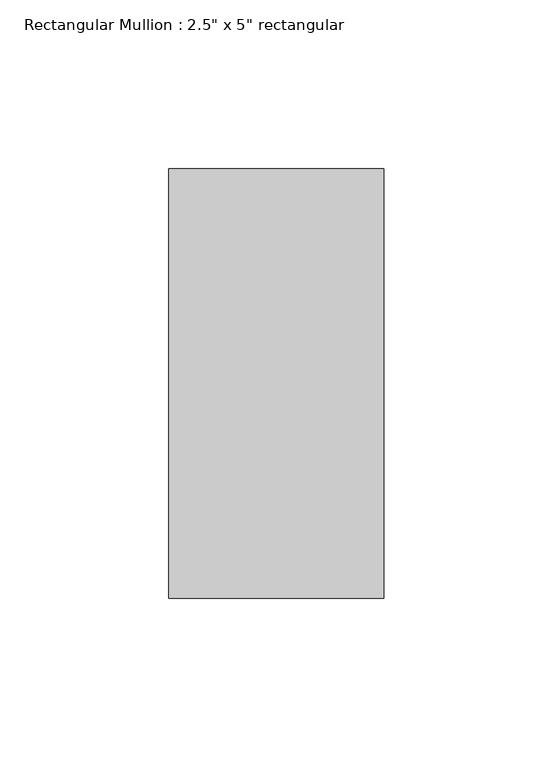
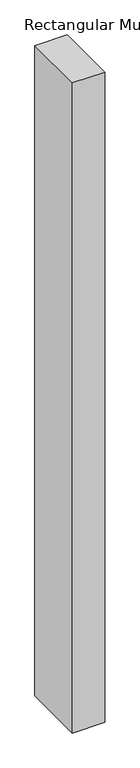
"""IFC4 building model written with IfcOpenShell, lengths in millimetres: member geometry."""

from ifc_helpers import new_model, si_unit, frame, origin, place, context, project, spatial, polyline, outline, extrude, source, transform, mapped, element, save


def member_488afbc6(model_context):
    return source(origin(), model_context, "Body", "SweptSolid", [
        extrude(outline(polyline([(31.75, 63.5), (31.75, -63.5), (-31.75, -63.5), (-31.75, 63.5), (31.75, 63.5)])), frame((0.0, 0.0, -1343.8279521), z_axis=(0.0, 0.0, 1.0), x_axis=(1.0, 0.0, 0.0)), (0.0, 0.0, 1.0), 1343.8279521),
    ])


if __name__ == "__main__":
    model = new_model("IFC4")
    model_context = context("Model", 3, world=origin())
    ifc_project = project(units=[si_unit("LENGTHUNIT", "METRE", prefix="MILLI")], contexts=[model_context])
    site = spatial("IfcSite", under=ifc_project)
    building = spatial("IfcBuilding", under=site)
    placement = place(None, origin())
    member_shape = member_488afbc6(model_context)
    element("IfcMember", 1, ObjectType="Rectangular Mullion : 2.5\" x 5\" rectangular", at=placement, inside=building, context=model_context, shape_type="MappedRepresentation", body=[
        mapped(member_shape, transform((0.0, 0.0, 0.0), x_axis=(1.0, 0.0, 0.0), y_axis=(0.0, 1.0, 0.0), z_axis=(0.0, 0.0, 1.0))),
    ])
    save(model, "model.ifc")

# Revit data of these elements
# Type "Rectangular Mullion : 2.5\" x 5\" rectangular"
#   built-in parameter 1007304 = 0.416667 (stored number, unit not read)
#   built-in parameter 1007301 = 0.104167 (stored number, unit not read)
#   built-in parameter 1007300 = 0.104167 (stored number, unit not read)
# Element 1 (IfcMember, "Rectangular Mullion : 2.5\" x 5\" rectangular")
#   Materials on its faces: "Aluminum"
# Materials
#   "Aluminum": class "Metal", colour RGB 247 247 247, transparency 0, Description = "Aluminum 6061", Cost = 0
